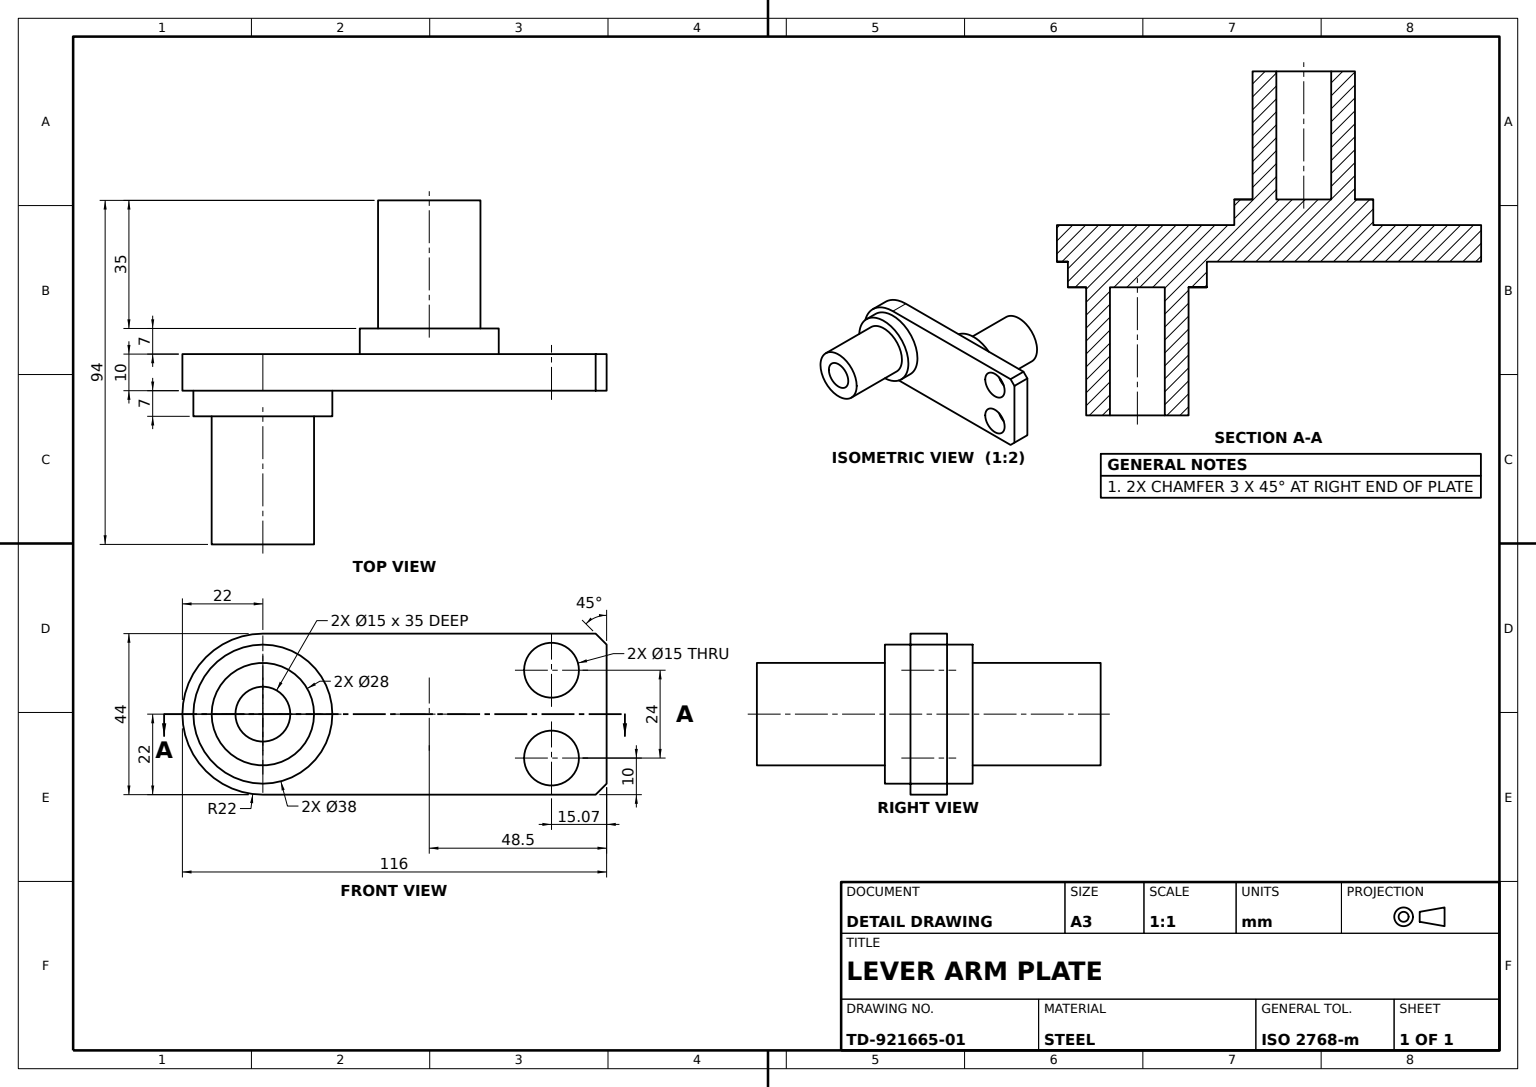
SolidWorks part; units mm, degrees
material "Plain Carbon Steel"
ref_plane "Front Plane" through (0, 0, 0) normal (0, 0, 1) x (1, 0, 0)
ref_plane "Top Plane" through (0, 0, 0) normal (0, 1, 0) x (1, 0, 0)
ref_plane "Right Plane" through (0, 0, 0) normal (1, 0, 0) x (0, 0, -1)
sketch "Base Plate Sketch" plane through (0, 0, 0) normal (0, 0, 1) x (1, 0, 0)
  line L0 (0, 22) -> (69, 22)
  line L1 (69, 22) -> (91, 22)
  line L2 (0, -22) -> (69, -22)
  line L3 (69, -22) -> (91, -22)
  line L8 (94, 19) -> (94, -19)
  line L9 (91, -22) -> (94, -19)
  line L10 (91, 22) -> (94, 19)
  arc A0 (0, 22) -> (0, -22) centre (0, 0) ccw
  dimension "D1" = 44
  dimension "D2" = 22
  dimension "D3" = 3
  dimension "D4" = 94
  dimension "D5" = 3
extrude "Base Plate" add sketch "Base Plate Sketch" along normal blind 10
sketch "Front Collar Sketch" plane through (0, 0, 10) normal (0, 0, 1) x (1, 0, 0)
  circle A0 centre (0, 0) radius 19
  dimension "D1" = 38
  dimension "D2" = 38
extrude "Front Collar Ø38" add sketch "Front Collar Sketch" along normal blind 7
sketch "Front Shaft Sketch" plane through (0, 0, 17) normal (0, 0, 1) x (1, 0, 0)
  circle A0 centre (0, 0) radius 14
  dimension "D1" = 28
  dimension "D2" = 28
extrude "Front Shaft Ø28" add sketch "Front Shaft Sketch" along normal blind 35
sketch "Rear Collar Sketch" plane through (0, 0, 0) normal (0, 0, -1) x (-1, 0, 0)
  line L0 (-91, 22) -> (0, 22) construction
  circle A0 centre (-45.5, 0) radius 19
  dimension "D1" = 38
  dimension "D2" = 38
  dimension "D3" = 48.5
  dimension "D4" = 22
extrude "Rear Collar Ø38" add sketch "Rear Collar Sketch" along normal blind 7
sketch "Rear Shaft Sketch" plane through (0, 0, -7) normal (0, 0, -1) x (-1, 0, 0)
  circle A0 centre (-45.5, 0) radius 14
  dimension "D1" = 28
  dimension "D2" = 28
extrude "Rear Shaft Ø28" add sketch "Rear Shaft Sketch" along normal blind 35
sketch "Rear Bore Sketch" plane through (0, 0, -42) normal (0, 0, -1) x (-1, 0, 0)
  circle A0 centre (-45.5, 0) radius 7.5
  dimension "D1" = 15
  dimension "D2" = 15
extrude "Rear Bore Ø15" cut sketch "Rear Bore Sketch" against normal blind 35
sketch "Front Bore Sketch" plane through (0, 0, 52) normal (0, 0, 1) x (1, 0, 0)
  circle A0 centre (0, 0) radius 7.5
  dimension "D1" = 15
  dimension "D2" = 15
extrude "Front Bore Ø15" cut sketch "Front Bore Sketch" against normal blind 35
sketch "End Holes Sketch" plane through (0, 0, 10) normal (0, 0, 1) x (1, 0, 0)
  line L0 (91, 22) -> (0, 22) construction
  line L1 (0, -22) -> (91, -22) construction
  circle A0 centre (78.9292, 12) radius 7.5
  circle A1 centre (78.9292, -12) radius 7.5
  dimension "D1" = 15
  dimension "D2" = 15
  dimension "D5" = 15
  dimension "D3" = 10
  dimension "D4" = 10
  dimension "D6" = 15.0708
extrude "End Holes 2xØ15" cut sketch "End Holes Sketch" against normal blind 10
